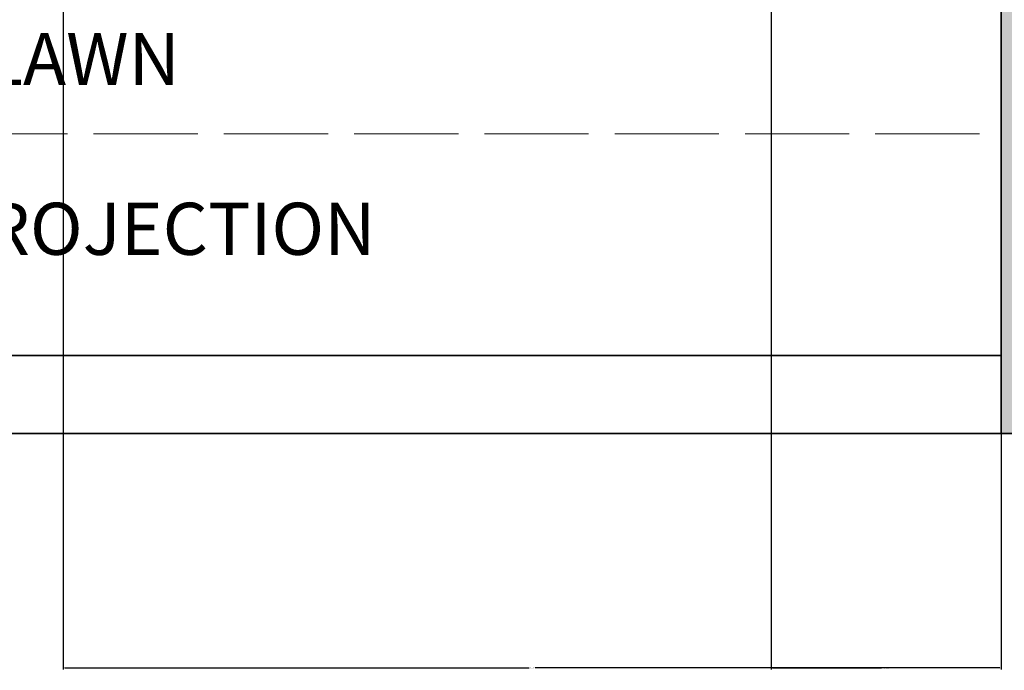
# Model space of a CAD drawing. Units: inches. Extents: x -5 to 330, y -522 to 40.
# Tile 13 of 23: x 159 to 272, y -522 to -447. Entities that reach past the tile are written whole.
import ezdxf

# ---------------------------------------------------------------- set-up
doc = ezdxf.new("R2010")
doc.units = ezdxf.units.IN
doc.header["$MEASUREMENT"] = 0
doc.linetypes.add('ACAD_ISO02W100', pattern=[15, 12, -3])
for name, color, linetype, lineweight in [('A-ANNO-DIMS', 2, 'Continuous', 18), ('A-ANNO-TEXT', 7, 'Continuous', 18), ('A-AREA-IDEN', 7, 'Continuous', 25), ('A-ROOF-OVHD', 8, 'ACAD_ISO02W100', 18), ('A-SITE-WALL', 7, 'Continuous', 35)]:
    doc.layers.add(name, color=color, linetype=linetype, lineweight=lineweight)
doc.layers.add('A-WALL-PATT', color=18, linetype='Continuous', lineweight=13, true_color=0x000000)
doc.styles.get("Standard").update_dxf_attribs({"font": 'arial.ttf'})
doc.dimstyles.get("Standard").update_dxf_attribs({"dimtxt": 0.18, "dimasz": 0.18, "dimexe": 0.18, "dimexo": 0.0625, "dimgap": 0.09, "dimtad": 0, "dimtih": 1, "dimtoh": 1, "dimdec": 0, "dimzin": 0, "dimdsep": 46, "dimlunit": 3, "dimtxsty": 'Standard', "dimcen": 0.09, "dimadec": 0, "dimazin": 0, "dimtfac": 1, "dimtdec": 0, "dimtofl": 0, "dimtmove": 0, "dimatfit": 3, "dimfxl": 1, "dimtolj": 1, "dimtzin": 0, "dimarcsym": 0})

# ---------------------------------------------------------------- blocks, each defined once
blk = doc.blocks.new('*D37')
at = {"layer": 'A-ANNO-DIMS', "color": 0, "lineweight": -2, "transparency": 16777216}
for p, q in [((164.01, -53.21), (164.01, -522.31)), ((272.01, -53.21), (272.01, -522.31)), ((164.19, -522.13), (217.68, -522.13)), ((271.83, -522.13), (218.34, -522.13))]:
    blk.add_line(p, q, dxfattribs=at)
at = {"layer": 'A-ANNO-DIMS', "color": 0, "transparency": 16777216}
for points in [[(164.19, -522.1), (164.19, -522.16), (164.01, -522.13)], [(271.83, -522.1), (271.83, -522.16), (272.01, -522.13)]]:
    blk.add_solid(points, dxfattribs=at)
at = {"layer": 'Defpoints', "color": 0, "transparency": 16777216}
for p in [(164.01, -53.14), (272.01, -53.14), (272.01, -522.13)]:
    blk.add_point(p, dxfattribs=at)
at = {"layer": 'A-ANNO-DIMS', "color": 0, "transparency": 16777216, "insert": (218.01, -522.13), "char_height": 0.18, "attachment_point": 5}
blk.add_mtext('\\A1;9\'-0"', dxfattribs=at)
blk = doc.blocks.new('*D46')
at = {"layer": 'A-ANNO-DIMS', "color": 0, "lineweight": -2, "transparency": 16777216}
for p, q in [((245.51, -426.21), (245.51, -522.31)), ((272.01, -426.21), (272.01, -522.31)), ((245.69, -522.13), (258.22, -522.13)), ((271.83, -522.13), (259.3, -522.13))]:
    blk.add_line(p, q, dxfattribs=at)
at = {"layer": 'A-ANNO-DIMS', "color": 0, "transparency": 16777216}
for points in [[(245.69, -522.1), (245.69, -522.16), (245.51, -522.13)], [(271.83, -522.1), (271.83, -522.16), (272.01, -522.13)]]:
    blk.add_solid(points, dxfattribs=at)
at = {"layer": 'Defpoints', "color": 0, "transparency": 16777216}
for p in [(245.51, -426.14), (272.01, -426.14), (272.01, -522.13)]:
    blk.add_point(p, dxfattribs=at)
at = {"layer": 'A-ANNO-DIMS', "color": 0, "transparency": 16777216, "insert": (258.76, -522.13), "char_height": 0.18, "attachment_point": 5}
blk.add_mtext('\\A1;2\'-2 1/2"', dxfattribs=at)

msp = doc.modelspace()

# ---------------------------------------------------------------- hatches: boundary and pattern name
at = {"layer": 'A-WALL-PATT'}
h = msp.add_hatch(color=256, dxfattribs=at)
h.dxf.hatch_style = 1
h.paths.add_polyline_path([(164.01, -44.15), (159.51, -44.15), (159.51, -153.14), (164.01, -153.14)], flags=17)
h.paths.add_polyline_path([(224.01, -188.14), (272.01, -188.14), (272.01, -218.14), (260.01, -218.14), (260.01, -222.64), (272.01, -222.64), (272.01, -292.64), (159.01, -292.64), (159.01, -297.14), (272.01, -297.14), (272.01, -417.14), (245.51, -417.14), (245.51, -426.14), (272.01, -426.14), (272.01, -495.14), (281.01, -495.14), (281.01, 12.36), (23.51, 12.36), (23.51, -426.14), (62.92, -426.14), (62.92, -417.14), (32.51, -417.14), (32.51, -297.14), (48.13, -297.14), (48.13, -292.64), (32.51, -292.64), (32.51, -140.64), (133.51, -140.64), (133.51, -131.64), (32.51, -131.64), (32.51, 3.36), (159.51, 3.36), (164.01, 3.36), (220.01, 3.36), (224.51, 3.36), (272.01, 3.36), (272.01, -179.14), (159.51, -179.14), (159.51, -188.14), (219.51, -188.14), (219.51, -266.64), (224.01, -266.64), (224.01, -222.64), (236.01, -222.64), (236.01, -218.14), (224.01, -218.14)])
h.paths.add_polyline_path([(133.01, -292.64), (128.51, -292.64), (128.51, -297.14), (128.51, -417.14), (122.92, -417.14), (122.92, -426.14), (133.01, -426.14)], flags=17)
h.paths.add_polyline_path([(185.51, -417.14), (159.01, -417.14), (159.01, -426.14), (185.51, -426.14)], flags=17)
h.paths.add_polyline_path([(133.51, -140.64), (129.01, -140.64), (129.01, -246.64), (133.51, -246.64)], flags=17)
h.paths.add_polyline_path([(246.01, -48.64), (224.51, -48.64), (224.51, -27.63), (220.01, -27.63), (220.01, -48.64), (198.6, -48.64), (198.6, -53.14), (246.01, -53.14)], flags=17)

# ---------------------------------------------------------------- linework, layer by layer
at = {"layer": 'A-ROOF-OVHD'}
msp.add_line((32.51, -460.64), (272.01, -460.64), dxfattribs=at)
at = {"layer": 'A-SITE-WALL'}
for p, q in [((272.01, -426.14), (272.01, -495.14)), ((128.36, -486.14), (272.01, -486.14)), ((23.51, -495.14), (281.01, -495.14))]:
    msp.add_line(p, q, dxfattribs=at)

# ---------------------------------------------------------------- texts
at = {"layer": 'A-ANNO-TEXT', "insert": (109.86, -468.56), "char_height": 6, "attachment_point": 1}
msp.add_mtext('3\'-6"WIDE PROJECTION', dxfattribs=at)
at = {"layer": 'A-AREA-IDEN', "insert": (126.49, -449.02), "char_height": 6, "attachment_point": 1}
msp.add_mtext('FRONT LAWN', dxfattribs=at)

# ---------------------------------------------------------------- dimensions: what is measured, and where the dimension line sits
at = {"layer": 'A-ANNO-DIMS'}
for p1, p2, picture, middle in [((164.01, -53.14), (272.01, -53.14), '*D37', (218.01, -522.13)), ((245.51, -426.14), (272.01, -426.14), '*D46', (258.76, -522.13))]:
    dim = msp.add_linear_dim(base=(272.01, -522.13), p1=p1, p2=p2, dimstyle='Standard', override={"dimdec": 1, "dimlfac": 1, "dimrnd": 0, "dimzin": 1, "dimdsep": 46, "dimlunit": 4, "dimfrac": 2}, dxfattribs=at)
    dim.commit()
    dim.dimension.update_dxf_attribs({"geometry": picture, "text_midpoint": middle})

doc.saveas('drawing.dxf')
